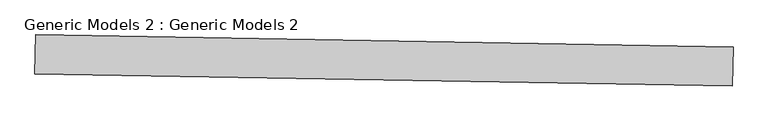
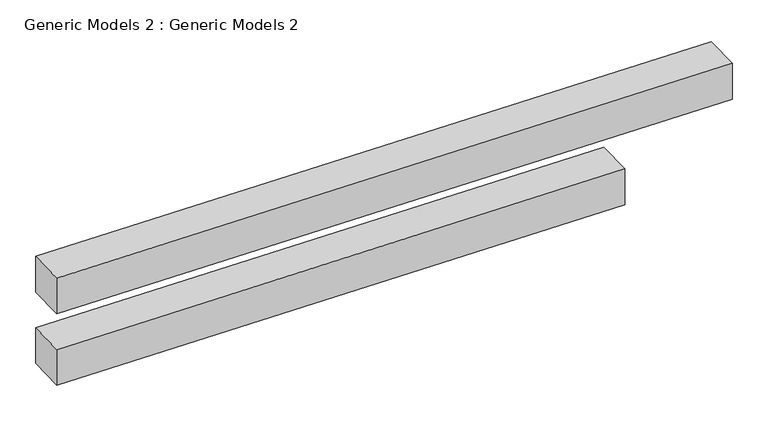
"""IFC4 building model written with IfcOpenShell, lengths in millimetres: proxy geometry, Generic Models 2 : Generic Models 2."""

from ifc_helpers import new_model, si_unit, frame, origin, place, context, project, spatial, polyline, outline, extrude, source, transform, mapped, element, save


def generic_models_2_generic_models_2_68b0420d(model_context):
    return source(origin(), model_context, "Body", "SweptSolid", [
        extrude(outline(polyline([(-3282.7051036, -11590.9636798), (-8696.2008129, -11496.4707607), (-8690.8813194, -11191.7171832), (-3277.3856101, -11286.2101023), (-3282.7051036, -11590.9636798)])), frame((0.0, 0.0, 938.3079965), z_axis=(0.0, 0.0, 1.0), x_axis=(1.0, 0.0, 0.0)), (0.0, 0.0, 1.0), 304.8),
        extrude(outline(polyline([(-4144.9829524, -11575.912564), (-8696.2008129, -11496.4707607), (-8690.8813194, -11191.7171832), (-4139.663459, -11271.1589865), (-4144.9829524, -11575.912564)])), frame((0.0, 0.0, 328.7079965), z_axis=(0.0, 0.0, 1.0), x_axis=(1.0, 0.0, 0.0)), (0.0, 0.0, 1.0), 304.8),
    ])


if __name__ == "__main__":
    model = new_model("IFC4")
    model_context = context("Model", 3, world=origin())
    ifc_project = project(units=[si_unit("LENGTHUNIT", "METRE", prefix="MILLI")], contexts=[model_context])
    site = spatial("IfcSite", under=ifc_project)
    building = spatial("IfcBuilding", under=site)
    placement = place(None, origin())
    generic_models_2_generic_models_2_shape = generic_models_2_generic_models_2_68b0420d(model_context)
    element("IfcBuildingElementProxy", 1, Name="Generic Models 2 : Generic Models 2", ObjectType="Generic Models 2 : Generic Models 2", at=placement, inside=building, context=model_context, shape_type="MappedRepresentation", body=[
        mapped(generic_models_2_generic_models_2_shape, transform((0.0, 0.0, 0.0), x_axis=(1.0, 0.0, 0.0), y_axis=(0.0, 1.0, 0.0), z_axis=(0.0, 0.0, 1.0))),
    ])
    save(model, "model.ifc")

# Revit data of these elements
# Element 1 (IfcBuildingElementProxy, "Generic Models 2 : Generic Models 2")
#   Materials on its faces: "Blanket"
# Materials
#   "Blanket": class "System", colour RGB 59 0 1, transparency 0, Cost = 0
